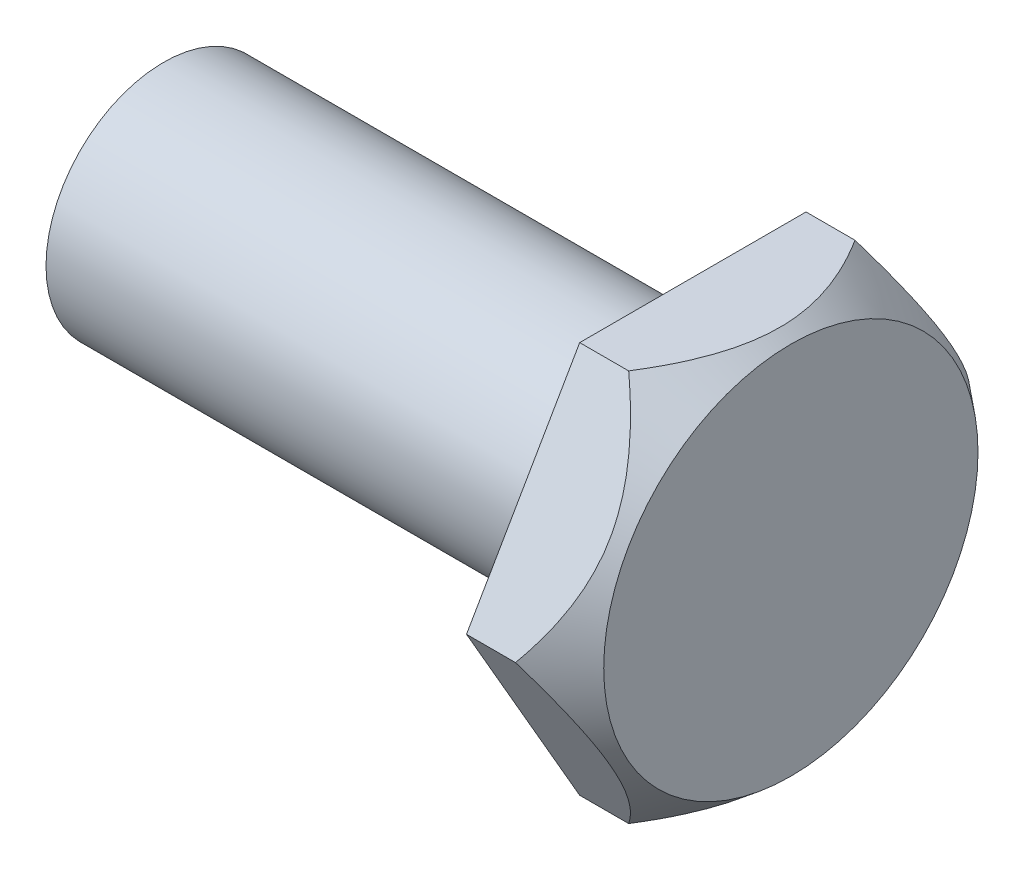
ISO-10303-21;
HEADER;
FILE_DESCRIPTION(('STEP AP214'),'2;1');
FILE_NAME('part.step','',(''),(''),'','','');
FILE_SCHEMA(('AUTOMOTIVE_DESIGN { 1 0 10303 214 1 1 1 1 }'));
ENDSEC;
DATA;
#1=APPLICATION_CONTEXT('core data for automotive mechanical design processes');
#2=APPLICATION_PROTOCOL_DEFINITION('international standard','automotive_design',2000,#1);
#3=PRODUCT_CONTEXT('',#1,'mechanical');
#4=PRODUCT('Part','Part','',(#3));
#5=PRODUCT_RELATED_PRODUCT_CATEGORY('part','',(#4));
#6=PRODUCT_DEFINITION_FORMATION('','',#4);
#7=PRODUCT_DEFINITION_CONTEXT('part definition',#1,'design');
#8=PRODUCT_DEFINITION('design','',#6,#7);
#9=PRODUCT_DEFINITION_SHAPE('','',#8);
#10=(LENGTH_UNIT() NAMED_UNIT(*) SI_UNIT(.MILLI.,.METRE.));
#11=(NAMED_UNIT(*) PLANE_ANGLE_UNIT() SI_UNIT($,.RADIAN.));
#12=(NAMED_UNIT(*) SI_UNIT($,.STERADIAN.) SOLID_ANGLE_UNIT());
#13=UNCERTAINTY_MEASURE_WITH_UNIT(LENGTH_MEASURE(1.E-05),#10,'distance_accuracy_value','');
#14=(GEOMETRIC_REPRESENTATION_CONTEXT(3) GLOBAL_UNCERTAINTY_ASSIGNED_CONTEXT((#13)) GLOBAL_UNIT_ASSIGNED_CONTEXT((#10,
#11,#12)) REPRESENTATION_CONTEXT('',''));
#15=CARTESIAN_POINT('',(0.,0.,0.));
#16=DIRECTION('',(0.,0.,1.));
#17=DIRECTION('',(1.,0.,0.));
#18=AXIS2_PLACEMENT_3D('',#15,#16,#17);
#19=CARTESIAN_POINT('',(5.,-9.99999999999994,-5.77350269189638));
#20=DIRECTION('',(0.,0.499999999999995,0.866025403784442));
#21=DIRECTION('',(0.,-0.866025403784442,0.499999999999995));
#22=AXIS2_PLACEMENT_3D('',#19,#20,#21);
#23=PLANE('',#22);
#24=CARTESIAN_POINT('',(2.49985566026766,-10.0001999999999,-5.77338722184254));
#25=CARTESIAN_POINT('',(2.60208467518783,-9.85852686353924,-5.85518224531506));
#26=CARTESIAN_POINT('',(2.70200639497535,-9.71558292882775,-5.93771096449977));
#27=CARTESIAN_POINT('',(2.89651431417004,-9.4269143562069,-6.104373842609));
#28=CARTESIAN_POINT('',(2.99109805277837,-9.28118847658979,-6.18850871843383));
#29=CARTESIAN_POINT('',(3.17470392595501,-8.98589768304951,-6.35899493757353));
#30=CARTESIAN_POINT('',(3.26368628893194,-8.83631408022678,-6.44535707092958));
#31=CARTESIAN_POINT('',(3.43446296157987,-8.53414647021996,-6.6198136219074));
#32=CARTESIAN_POINT('',(3.51625815008562,-8.38156283267477,-6.70790782611805));
#33=CARTESIAN_POINT('',(3.75045112758238,-7.91690475517259,-6.97617829224507));
#34=CARTESIAN_POINT('',(3.89039553403278,-7.59990272498793,-7.15919949970583));
#35=CARTESIAN_POINT('',(4.06799913309065,-7.1160294270294,-7.43856387853586));
#36=CARTESIAN_POINT('',(4.12177377354539,-6.95352485751446,-7.53238593548985));
#37=CARTESIAN_POINT('',(4.21746692388596,-6.62593053507777,-7.72152260573366));
#38=CARTESIAN_POINT('',(4.25938815721112,-6.46084138520395,-7.8168368708536));
#39=CARTESIAN_POINT('',(4.33871032958248,-6.08911976471419,-8.03145044850696));
#40=CARTESIAN_POINT('',(4.37267748881161,-5.88192616358385,-8.15107372989393));
#41=CARTESIAN_POINT('',(4.41927948249989,-5.46569987173225,-8.39138209153825));
#42=CARTESIAN_POINT('',(4.43191113799902,-5.25666691161239,-8.51206732733295));
#43=CARTESIAN_POINT('',(4.43521434084648,-4.83984013132415,-8.75272238113781));
#44=CARTESIAN_POINT('',(4.42602965332971,-4.63204719513949,-8.87269168877972));
#45=CARTESIAN_POINT('',(4.38644510874876,-4.21800376920535,-9.11173977219899));
#46=CARTESIAN_POINT('',(4.35604439850546,-4.0117533418233,-9.23081851196849));
#47=CARTESIAN_POINT('',(4.26630141702067,-3.55618197525321,-9.49384276309281));
#48=CARTESIAN_POINT('',(4.20199147726657,-3.30759485824364,-9.63736460201536));
#49=CARTESIAN_POINT('',(4.04725502781986,-2.8165969751545,-9.92084236198841));
#50=CARTESIAN_POINT('',(3.95681699311202,-2.57418898612793,-10.0607966797066));
#51=CARTESIAN_POINT('',(3.75343720990721,-2.09504523404485,-10.3374304539523));
#52=CARTESIAN_POINT('',(3.64036752653577,-1.85835070482231,-10.4740861041146));
#53=CARTESIAN_POINT('',(3.39608726520655,-1.39222410263783,-10.7432044233623));
#54=CARTESIAN_POINT('',(3.26488079551853,-1.1627903994069,-10.8756680336838));
#55=CARTESIAN_POINT('',(3.02822583050869,-0.776777620154309,-11.098532615696));
#56=CARTESIAN_POINT('',(2.92644536946085,-0.618490041669188,-11.1899199917437));
#57=CARTESIAN_POINT('',(2.71725475169805,-0.306260702457589,-11.3701856847864));
#58=CARTESIAN_POINT('',(2.60989089909902,-0.152295714503421,-11.4590774120275));
#59=CARTESIAN_POINT('',(2.49985566026766,0.00019999999999962,-11.5471208538464));
#60=B_SPLINE_CURVE_WITH_KNOTS('',3,(#24,#25,#26,#27,#28,#29,#30,#31,#32,#33,#34,#35,#36,#37,#38,
#39,#40,#41,#42,#43,#44,#45,#46,#47,#48,#49,#50,#51,#52,#53,#54,#55,#56,#57,#58,#59),
.UNSPECIFIED.,.F.,.F.,(4,2,2,2,2,2,2,2,2,2,2,2,2,2,2,2,2,4),(0.,0.578726598225102,
1.15771784486318,1.74044053909011,2.32309187958723,3.49620252422061,4.08148401745194,
4.66663092690834,5.39064458743798,6.11476611547105,6.83412908628144,7.55352098715262,
8.43453361817369,9.31593545579789,10.2024681456462,11.0888003498481,11.7162856672066,
12.3392094455715),.UNSPECIFIED.);
#61=CARTESIAN_POINT('',(2.5,-9.99999999999994,-5.77350269189637));
#62=VERTEX_POINT('',#61);
#63=CARTESIAN_POINT('',(2.5,0.,-11.5470053837925));
#64=VERTEX_POINT('',#63);
#65=EDGE_CURVE('E145',#62,#64,#60,.T.);
#66=ORIENTED_EDGE('',*,*,#65,.F.);
#67=DIRECTION('',(-1.,0.,0.));
#68=VECTOR('',#67,1.);
#69=CARTESIAN_POINT('',(5.,-9.99999999999994,-5.77350269189638));
#70=LINE('',#69,#68);
#71=CARTESIAN_POINT('',(0.,-9.99999999999994,-5.77350269189638));
#72=VERTEX_POINT('',#71);
#73=EDGE_CURVE('E64',#62,#72,#70,.T.);
#74=ORIENTED_EDGE('',*,*,#73,.T.);
#75=DIRECTION('',(0.,0.866025403784442,-0.499999999999995));
#76=VECTOR('',#75,1.);
#77=CARTESIAN_POINT('',(0.,-9.99999999999994,-5.77350269189638));
#78=LINE('',#77,#76);
#79=CARTESIAN_POINT('',(0.,0.,-11.5470053837925));
#80=VERTEX_POINT('',#79);
#81=EDGE_CURVE('E137',#72,#80,#78,.T.);
#82=ORIENTED_EDGE('',*,*,#81,.T.);
#83=DIRECTION('',(-1.,0.,0.));
#84=VECTOR('',#83,1.);
#85=CARTESIAN_POINT('',(5.,0.,-11.5470053837925));
#86=LINE('',#85,#84);
#87=EDGE_CURVE('E43',#64,#80,#86,.T.);
#88=ORIENTED_EDGE('',*,*,#87,.F.);
#89=EDGE_LOOP('',(#66,#74,#82,#88));
#90=FACE_BOUND('',#89,.T.);
#91=ADVANCED_FACE('F39',(#90),#23,.F.);
#92=CARTESIAN_POINT('',(5.,0.,-11.5470053837925));
#93=DIRECTION('',(0.,-0.500000000000001,0.866025403784438));
#94=DIRECTION('',(0.,-0.866025403784438,-0.500000000000001));
#95=AXIS2_PLACEMENT_3D('',#92,#93,#94);
#96=PLANE('',#95);
#97=CARTESIAN_POINT('',(2.49985566026766,-0.000200000000000101,-11.5471208538464));
#98=CARTESIAN_POINT('',(2.60208467518784,0.141473136460705,-11.4653258303738));
#99=CARTESIAN_POINT('',(2.70200639497536,0.284417071172192,-11.3827971111891));
#100=CARTESIAN_POINT('',(2.89651431417006,0.57308564379305,-11.2161342330799));
#101=CARTESIAN_POINT('',(2.99109805277838,0.718811523410157,-11.1319993572551));
#102=CARTESIAN_POINT('',(3.17470392595503,1.01410231695044,-10.9615131381154));
#103=CARTESIAN_POINT('',(3.26368628893196,1.16368591977317,-10.8751510047593));
#104=CARTESIAN_POINT('',(3.43446296157989,1.46585352977999,-10.7006944537815));
#105=CARTESIAN_POINT('',(3.51625815008564,1.61843716732518,-10.6126002495708));
#106=CARTESIAN_POINT('',(3.75045112758241,2.08309524482737,-10.3443297834438));
#107=CARTESIAN_POINT('',(3.89039553403281,2.40009727501203,-10.161308575983));
#108=CARTESIAN_POINT('',(4.06799913309069,2.88397057297057,-9.881944197153));
#109=CARTESIAN_POINT('',(4.12177377354543,3.04647514248551,-9.78812214019901));
#110=CARTESIAN_POINT('',(4.217466923886,3.37406946492221,-9.59898546995518));
#111=CARTESIAN_POINT('',(4.25938815721117,3.53915861479603,-9.50367120483525));
#112=CARTESIAN_POINT('',(4.33871032958253,3.91088023528579,-9.28905762718188));
#113=CARTESIAN_POINT('',(4.37267748881166,4.11807383641612,-9.16943434579491));
#114=CARTESIAN_POINT('',(4.41927948249994,4.53430012826773,-8.92912598415059));
#115=CARTESIAN_POINT('',(4.43191113799907,4.74333308838758,-8.80844074835589));
#116=CARTESIAN_POINT('',(4.43521434084653,5.16015986867583,-8.56778569455102));
#117=CARTESIAN_POINT('',(4.42602965332976,5.36795280486048,-8.44781638690911));
#118=CARTESIAN_POINT('',(4.38644510874881,5.78199623079462,-8.20876830348984));
#119=CARTESIAN_POINT('',(4.35604439850552,5.98824665817666,-8.08968956372034));
#120=CARTESIAN_POINT('',(4.26630141702072,6.44381802474675,-7.82666531259602));
#121=CARTESIAN_POINT('',(4.20199147726662,6.69240514175632,-7.68314347367347));
#122=CARTESIAN_POINT('',(4.04725502781991,7.18340302484546,-7.39966571370041));
#123=CARTESIAN_POINT('',(3.95681699311207,7.42581101387203,-7.25971139598221));
#124=CARTESIAN_POINT('',(3.75343720990726,7.9049547659551,-6.98307762173652));
#125=CARTESIAN_POINT('',(3.64036752653582,8.14164929517764,-6.84642197157417));
#126=CARTESIAN_POINT('',(3.3960872652066,8.60777589736212,-6.57730365232652));
#127=CARTESIAN_POINT('',(3.26488079551859,8.83720960059305,-6.44484004200497));
#128=CARTESIAN_POINT('',(3.02822583050874,9.22322237984565,-6.22197545999284));
#129=CARTESIAN_POINT('',(2.92644536946089,9.38150995833078,-6.13058808394508));
#130=CARTESIAN_POINT('',(2.71725475169808,9.69373929754241,-5.95032239090235));
#131=CARTESIAN_POINT('',(2.60989089909903,9.84770428549659,-5.86143066366122));
#132=CARTESIAN_POINT('',(2.49985566026766,10.0002,-5.7733872218424));
#133=B_SPLINE_CURVE_WITH_KNOTS('',3,(#97,#98,#99,#100,#101,#102,#103,#104,#105,#106,#107,#108,
#109,#110,#111,#112,#113,#114,#115,#116,#117,#118,#119,#120,#121,#122,#123,#124,#125,#126,#127,
#128,#129,#130,#131,#132),.UNSPECIFIED.,.F.,.F.,(4,2,2,2,2,2,2,2,2,2,2,2,2,2,2,2,2,4),(0.,
0.578726598225111,1.1577178448632,1.74044053909014,2.32309187958726,3.49620252422066,
4.081484017452,4.66663092690841,5.39064458743805,6.11476611547112,6.83412908628151,
7.55352098715269,8.43453361817375,9.31593545579795,10.2024681456462,11.0888003498482,
11.7162856672067,12.3392094455717),.UNSPECIFIED.);
#134=CARTESIAN_POINT('',(2.5,10.,-5.77350269189624));
#135=VERTEX_POINT('',#134);
#136=EDGE_CURVE('E131',#64,#135,#133,.T.);
#137=ORIENTED_EDGE('',*,*,#136,.F.);
#138=ORIENTED_EDGE('',*,*,#87,.T.);
#139=DIRECTION('',(0.,0.866025403784438,0.500000000000001));
#140=VECTOR('',#139,1.);
#141=CARTESIAN_POINT('',(0.,0.,-11.5470053837925));
#142=LINE('',#141,#140);
#143=CARTESIAN_POINT('',(0.,10.,-5.77350269189624));
#144=VERTEX_POINT('',#143);
#145=EDGE_CURVE('E126',#80,#144,#142,.T.);
#146=ORIENTED_EDGE('',*,*,#145,.T.);
#147=DIRECTION('',(-1.,0.,0.));
#148=VECTOR('',#147,1.);
#149=CARTESIAN_POINT('',(5.,10.,-5.77350269189624));
#150=LINE('',#149,#148);
#151=EDGE_CURVE('E116',#135,#144,#150,.T.);
#152=ORIENTED_EDGE('',*,*,#151,.F.);
#153=EDGE_LOOP('',(#137,#138,#146,#152));
#154=FACE_BOUND('',#153,.T.);
#155=ADVANCED_FACE('F129',(#154),#96,.F.);
#156=CARTESIAN_POINT('',(5.,10.,-5.77350269189624));
#157=DIRECTION('',(0.,-1.,0.));
#158=DIRECTION('',(0.,0.,-1.));
#159=AXIS2_PLACEMENT_3D('',#156,#157,#158);
#160=PLANE('',#159);
#161=CARTESIAN_POINT('',(-8.35662706903642,10.0000000000001,-17.5882417575278));
#162=CARTESIAN_POINT('',(-7.97728774264987,10.0000000000001,-17.2391089345561));
#163=CARTESIAN_POINT('',(-7.59917023824418,10.0000000000001,-16.888638172075));
#164=CARTESIAN_POINT('',(-6.84592339805097,10.0000000000001,-16.1844494205654));
#165=CARTESIAN_POINT('',(-6.4707942720274,10.0000000000001,-15.8307312072743));
#166=CARTESIAN_POINT('',(-5.72329920958807,10.,-15.1187412536086));
#167=CARTESIAN_POINT('',(-5.3509411810078,10.,-14.7604611985171));
#168=CARTESIAN_POINT('',(-4.61061924843071,10.,-14.0394023341909));
#169=CARTESIAN_POINT('',(-4.24265522995826,10.,-13.6766236426619));
#170=CARTESIAN_POINT('',(-3.50698481181781,10.,-12.9405134735512));
#171=CARTESIAN_POINT('',(-3.1393549670149,10.,-12.5671053329458));
#172=CARTESIAN_POINT('',(-2.41108252260193,10.,-11.8135408542725));
#173=CARTESIAN_POINT('',(-2.05043969112774,10.,-11.4333847409411));
#174=CARTESIAN_POINT('',(-1.33839051853618,10.,-10.6650878734714));
#175=CARTESIAN_POINT('',(-0.986976669328572,10.,-10.2769540985743));
#176=CARTESIAN_POINT('',(-0.295851771817263,10.,-9.49043781030286));
#177=CARTESIAN_POINT('',(0.0438610505675598,10.,-9.09205686672108));
#178=CARTESIAN_POINT('',(0.607339330625165,10.,-8.40467587052712));
#179=CARTESIAN_POINT('',(0.835132848513796,10.,-8.11898389461643));
#180=CARTESIAN_POINT('',(1.28117912364746,10.,-7.54016134039821));
#181=CARTESIAN_POINT('',(1.49943087980217,10.,-7.24702998665042));
#182=CARTESIAN_POINT('',(1.92390022086966,10.,-6.65199419820068));
#183=CARTESIAN_POINT('',(2.13011400830235,10.,-6.35008703960652));
#184=CARTESIAN_POINT('',(2.52701179015707,10.,-5.73618278704565));
#185=CARTESIAN_POINT('',(2.71769748897819,10.,-5.42418680571781));
#186=CARTESIAN_POINT('',(3.05280570259878,10.,-4.83469068446123));
#187=CARTESIAN_POINT('',(3.19992926298762,10.,-4.55873561198774));
#188=CARTESIAN_POINT('',(3.47579299967202,10.,-3.99765646875701));
#189=CARTESIAN_POINT('',(3.60453166636243,10.,-3.71253164741337));
#190=CARTESIAN_POINT('',(3.8387515987253,10.,-3.13389541890926));
#191=CARTESIAN_POINT('',(3.94430995674006,10.,-2.84041559417784));
#192=CARTESIAN_POINT('',(4.12772031764736,10.,-2.24490150142743));
#193=CARTESIAN_POINT('',(4.20558602056865,10.,-1.94287154337203));
#194=CARTESIAN_POINT('',(4.31392399550829,10.,-1.40660042017346));
#195=CARTESIAN_POINT('',(4.35131898505701,10.,-1.17375444581952));
#196=CARTESIAN_POINT('',(4.40605033394989,10.,-0.705707397152917));
#197=CARTESIAN_POINT('',(4.42338948717618,10.,-0.47050665547711));
#198=CARTESIAN_POINT('',(4.43721854881449,10.,0.000395911575754617));
#199=CARTESIAN_POINT('',(4.43371867902631,10.,0.236097434604736));
#200=CARTESIAN_POINT('',(4.40605758957446,10.,0.706283855006258));
#201=CARTESIAN_POINT('',(4.38189519433181,10.,0.940768682392127));
#202=CARTESIAN_POINT('',(4.31417340982602,9.99999999999999,1.40551529862139));
#203=CARTESIAN_POINT('',(4.27072569970184,9.99999999999999,1.63579356640222));
#204=CARTESIAN_POINT('',(4.16615955139027,9.99999999999999,2.09231382275418));
#205=CARTESIAN_POINT('',(4.1050370725345,9.99999999999999,2.31855487579778));
#206=CARTESIAN_POINT('',(3.9670838088809,9.99999999999999,2.76646805689877));
#207=CARTESIAN_POINT('',(3.89023306874717,9.99999999999999,2.98813398298915));
#208=CARTESIAN_POINT('',(3.72298819408545,9.99999999999999,3.42624280728566));
#209=CARTESIAN_POINT('',(3.63259437104085,9.99999999999999,3.64268582548288));
#210=CARTESIAN_POINT('',(3.40888186338885,9.99999999999999,4.14008164597385));
#211=CARTESIAN_POINT('',(3.27117741048021,9.99999999999998,4.41905695199646));
#212=CARTESIAN_POINT('',(2.97942567580929,9.99999999999998,4.96838107495215));
#213=CARTESIAN_POINT('',(2.82537119433022,9.99999999999998,5.23872602278562));
#214=CARTESIAN_POINT('',(2.50391254127959,9.99999999999998,5.7719758553274));
#215=CARTESIAN_POINT('',(2.33648474477565,9.99999999999998,6.03486640976312));
#216=CARTESIAN_POINT('',(1.99111175713331,9.99999999999998,6.55355223906987));
#217=CARTESIAN_POINT('',(1.81316801950844,9.99999999999998,6.80934848736804));
#218=CARTESIAN_POINT('',(1.44673171699159,9.99999999999998,7.31752860399921));
#219=CARTESIAN_POINT('',(1.25814474063016,9.99999999999998,7.56984411339175));
#220=CARTESIAN_POINT('',(0.873829840215399,9.99999999999997,8.06896766590264));
#221=CARTESIAN_POINT('',(0.678101729330905,9.99999999999997,8.31577556465454));
#222=CARTESIAN_POINT('',(0.280957134366479,9.99999999999997,8.80434376141056));
#223=CARTESIAN_POINT('',(0.0795466103589055,9.99999999999997,9.04610891705088));
#224=CARTESIAN_POINT('',(-0.328183318593257,9.99999999999997,9.52546854557073));
#225=CARTESIAN_POINT('',(-0.534502903544672,9.99999999999997,9.76306286495601));
#226=CARTESIAN_POINT('',(-1.04494842355568,9.99999999999997,10.3406073190432));
#227=CARTESIAN_POINT('',(-1.35134375872624,9.99999999999997,10.6785507196934));
#228=CARTESIAN_POINT('',(-1.9709756821915,9.99999999999996,11.3481047128741));
#229=CARTESIAN_POINT('',(-2.28421252369331,9.99999999999996,11.6797150701615));
#230=CARTESIAN_POINT('',(-2.91635203293325,9.99999999999996,12.337808130985));
#231=CARTESIAN_POINT('',(-3.23525752273593,9.99999999999996,12.6642881188828));
#232=CARTESIAN_POINT('',(-3.87757020644268,9.99999999999996,13.3127893326489));
#233=CARTESIAN_POINT('',(-4.20097745572092,9.99999999999995,13.6348105035737));
#234=CARTESIAN_POINT('',(-4.83999412661594,9.99999999999995,14.2637274750938));
#235=CARTESIAN_POINT('',(-5.15547404837216,9.99999999999995,14.5707550365838));
#236=CARTESIAN_POINT('',(-5.78935532002772,9.99999999999995,15.1817824119234));
#237=CARTESIAN_POINT('',(-6.10775669613608,9.99999999999995,15.4857821985592));
#238=CARTESIAN_POINT('',(-6.74669312096204,9.99999999999995,16.0908355033313));
#239=CARTESIAN_POINT('',(-7.0672254987366,9.99999999999995,16.3918918449499));
#240=CARTESIAN_POINT('',(-7.71041486444918,9.99999999999994,16.9917064317293));
#241=CARTESIAN_POINT('',(-8.03307178396953,9.99999999999994,17.2904647502292));
#242=CARTESIAN_POINT('',(-8.35662706903642,9.99999999999994,17.5882417575279));
#243=B_SPLINE_CURVE_WITH_KNOTS('',3,(#161,#162,#163,#164,#165,#166,#167,#168,#169,#170,#171,
#172,#173,#174,#175,#176,#177,#178,#179,#180,#181,#182,#183,#184,#185,#186,#187,#188,#189,#190,
#191,#192,#193,#194,#195,#196,#197,#198,#199,#200,#201,#202,#203,#204,#205,#206,#207,#208,#209,
#210,#211,#212,#213,#214,#215,#216,#217,#218,#219,#220,#221,#222,#223,#224,#225,#226,#227,#228,
#229,#230,#231,#232,#233,#234,#235,#236,#237,#238,#239,#240,#241,#242),.UNSPECIFIED.,.F.,.F.,(4,
2,2,2,2,2,2,2,2,2,2,2,2,2,2,2,2,2,2,2,2,2,2,2,2,2,2,2,2,2,2,2,2,2,2,2,2,2,2,2,4),(0.,
1.54665805225938,3.09342372941361,4.64359691339925,6.19372962276105,7.7656852884161,
9.33758869903942,10.9081709990313,12.4785141134674,13.5745278278695,14.6706562578265,
15.7671286227889,16.8634804737197,17.8011113362478,18.7388191445309,19.6733594653186,
20.6074368078336,21.3141402405969,22.0207452140419,22.727003617527,23.4333022057311,
24.1355629998527,24.8379844664794,25.5413027222289,26.244604804531,27.1772291450048,
28.1102658830341,29.0449889881248,29.979583196587,30.9244446421433,31.8693308255509,
32.8132603206112,33.7572244814476,35.1255826710275,36.4939915902383,37.8631019732006,
39.2322292118992,40.552865604745,41.8735138569189,43.192738059353,44.5119199839387),.UNSPECIFIED.);
#244=CARTESIAN_POINT('',(2.5,9.99999999999998,5.77350269189631));
#245=VERTEX_POINT('',#244);
#246=EDGE_CURVE('E98',#135,#245,#243,.T.);
#247=ORIENTED_EDGE('',*,*,#246,.F.);
#248=ORIENTED_EDGE('',*,*,#151,.T.);
#249=DIRECTION('',(0.,0.,1.));
#250=VECTOR('',#249,1.);
#251=CARTESIAN_POINT('',(0.,10.,-5.77350269189624));
#252=LINE('',#251,#250);
#253=CARTESIAN_POINT('',(0.,9.99999999999998,5.77350269189631));
#254=VERTEX_POINT('',#253);
#255=EDGE_CURVE('E140',#144,#254,#252,.T.);
#256=ORIENTED_EDGE('',*,*,#255,.T.);
#257=DIRECTION('',(-1.,0.,0.));
#258=VECTOR('',#257,1.);
#259=CARTESIAN_POINT('',(5.,9.99999999999998,5.77350269189631));
#260=LINE('',#259,#258);
#261=EDGE_CURVE('E112',#245,#254,#260,.T.);
#262=ORIENTED_EDGE('',*,*,#261,.F.);
#263=EDGE_LOOP('',(#247,#248,#256,#262));
#264=FACE_BOUND('',#263,.T.);
#265=ADVANCED_FACE('F201',(#264),#160,.F.);
#266=CARTESIAN_POINT('',(5.,9.99999999999998,5.77350269189631));
#267=DIRECTION('',(0.,-0.499999999999995,-0.866025403784442));
#268=DIRECTION('',(0.,0.866025403784442,-0.499999999999995));
#269=AXIS2_PLACEMENT_3D('',#266,#267,#268);
#270=PLANE('',#269);
#271=CARTESIAN_POINT('',(2.49985566026766,10.0002,5.77338722184247));
#272=CARTESIAN_POINT('',(2.60208467518784,9.85852686353928,5.855182245315));
#273=CARTESIAN_POINT('',(2.70200639497535,9.71558292882779,5.9377109644997));
#274=CARTESIAN_POINT('',(2.89651431417006,9.42691435620693,6.10437384260893));
#275=CARTESIAN_POINT('',(2.99109805277838,9.28118847658982,6.18850871843376));
#276=CARTESIAN_POINT('',(3.17470392595502,8.98589768304953,6.35899493757346));
#277=CARTESIAN_POINT('',(3.26368628893196,8.83631408022681,6.44535707092952));
#278=CARTESIAN_POINT('',(3.43446296157989,8.53414647021998,6.61981362190734));
#279=CARTESIAN_POINT('',(3.51625815008564,8.3815628326748,6.70790782611799));
#280=CARTESIAN_POINT('',(3.75045112758241,7.9169047551726,6.97617829224501));
#281=CARTESIAN_POINT('',(3.89039553403281,7.59990272498794,7.15919949970578));
#282=CARTESIAN_POINT('',(4.06799913309069,7.11602942702941,7.43856387853581));
#283=CARTESIAN_POINT('',(4.12177377354543,6.95352485751446,7.5323859354898));
#284=CARTESIAN_POINT('',(4.217466923886,6.62593053507777,7.72152260573362));
#285=CARTESIAN_POINT('',(4.25938815721116,6.46084138520394,7.81683687085356));
#286=CARTESIAN_POINT('',(4.33871032958253,6.08911976471418,8.03145044850692));
#287=CARTESIAN_POINT('',(4.37267748881166,5.88192616358385,8.15107372989389));
#288=CARTESIAN_POINT('',(4.41927948249994,5.46569987173224,8.3913820915382));
#289=CARTESIAN_POINT('',(4.43191113799907,5.25666691161239,8.51206732733291));
#290=CARTESIAN_POINT('',(4.43521434084653,4.83984013132414,8.75272238113777));
#291=CARTESIAN_POINT('',(4.42602965332976,4.63204719513949,8.87269168877968));
#292=CARTESIAN_POINT('',(4.38644510874881,4.21800376920535,9.11173977219895));
#293=CARTESIAN_POINT('',(4.35604439850552,4.0117533418233,9.23081851196844));
#294=CARTESIAN_POINT('',(4.26630141702072,3.55618197525321,9.49384276309277));
#295=CARTESIAN_POINT('',(4.20199147726662,3.30759485824364,9.63736460201532));
#296=CARTESIAN_POINT('',(4.04725502781991,2.81659697515451,9.92084236198836));
#297=CARTESIAN_POINT('',(3.95681699311208,2.57418898612793,10.0607966797066));
#298=CARTESIAN_POINT('',(3.75343720990727,2.09504523404486,10.3374304539523));
#299=CARTESIAN_POINT('',(3.64036752653583,1.85835070482232,10.4740861041146));
#300=CARTESIAN_POINT('',(3.39608726520661,1.39222410263784,10.7432044233622));
#301=CARTESIAN_POINT('',(3.26488079551859,1.16279039940691,10.8756680336838));
#302=CARTESIAN_POINT('',(3.02822583050874,0.776777620154306,11.0985326156959));
#303=CARTESIAN_POINT('',(2.92644536946089,0.618490041669168,11.1899199917437));
#304=CARTESIAN_POINT('',(2.71725475169808,0.306260702457537,11.3701856847864));
#305=CARTESIAN_POINT('',(2.60989089909903,0.152295714503355,11.4590774120275));
#306=CARTESIAN_POINT('',(2.49985566026766,-0.000200000000078887,11.5471208538464));
#307=B_SPLINE_CURVE_WITH_KNOTS('',3,(#271,#272,#273,#274,#275,#276,#277,#278,#279,#280,#281,
#282,#283,#284,#285,#286,#287,#288,#289,#290,#291,#292,#293,#294,#295,#296,#297,#298,#299,#300,
#301,#302,#303,#304,#305,#306),.UNSPECIFIED.,.F.,.F.,(4,2,2,2,2,2,2,2,2,2,2,2,2,2,2,2,2,4),(0.,
0.578726598225112,1.1577178448632,1.74044053909014,2.32309187958726,3.49620252422066,
4.081484017452,4.66663092690841,5.39064458743804,6.11476611547111,6.83412908628151,
7.55352098715268,8.43453361817375,9.31593545579794,10.2024681456462,11.0888003498482,
11.7162856672067,12.3392094455717),.UNSPECIFIED.);
#308=CARTESIAN_POINT('',(2.5,0.,11.5470053837925));
#309=VERTEX_POINT('',#308);
#310=EDGE_CURVE('E94',#245,#309,#307,.T.);
#311=ORIENTED_EDGE('',*,*,#310,.F.);
#312=ORIENTED_EDGE('',*,*,#261,.T.);
#313=DIRECTION('',(0.,-0.866025403784442,0.499999999999995));
#314=VECTOR('',#313,1.);
#315=CARTESIAN_POINT('',(0.,9.99999999999998,5.77350269189631));
#316=LINE('',#315,#314);
#317=CARTESIAN_POINT('',(0.,0.,11.5470053837925));
#318=VERTEX_POINT('',#317);
#319=EDGE_CURVE('E115',#254,#318,#316,.T.);
#320=ORIENTED_EDGE('',*,*,#319,.T.);
#321=DIRECTION('',(-1.,0.,0.));
#322=VECTOR('',#321,1.);
#323=CARTESIAN_POINT('',(5.,0.,11.5470053837925));
#324=LINE('',#323,#322);
#325=EDGE_CURVE('E102',#309,#318,#324,.T.);
#326=ORIENTED_EDGE('',*,*,#325,.F.);
#327=EDGE_LOOP('',(#311,#312,#320,#326));
#328=FACE_BOUND('',#327,.T.);
#329=ADVANCED_FACE('F109',(#328),#270,.F.);
#330=CARTESIAN_POINT('',(5.,0.,11.5470053837925));
#331=DIRECTION('',(0.,0.500000000000007,-0.866025403784435));
#332=DIRECTION('',(0.,0.866025403784435,0.500000000000007));
#333=AXIS2_PLACEMENT_3D('',#330,#331,#332);
#334=PLANE('',#333);
#335=CARTESIAN_POINT('',(2.49985566026766,0.000199999999919467,11.5471208538464));
#336=CARTESIAN_POINT('',(2.60208467518784,-0.141473136460786,11.4653258303738));
#337=CARTESIAN_POINT('',(2.70200639497535,-0.284417071172273,11.3827971111891));
#338=CARTESIAN_POINT('',(2.89651431417006,-0.573085643793129,11.2161342330799));
#339=CARTESIAN_POINT('',(2.99109805277838,-0.718811523410235,11.1319993572551));
#340=CARTESIAN_POINT('',(3.17470392595503,-1.01410231695052,10.9615131381154));
#341=CARTESIAN_POINT('',(3.26368628893196,-1.16368591977324,10.8751510047593));
#342=CARTESIAN_POINT('',(3.43446296157989,-1.46585352978007,10.7006944537815));
#343=CARTESIAN_POINT('',(3.51625815008564,-1.61843716732525,10.6126002495708));
#344=CARTESIAN_POINT('',(3.75045112758241,-2.08309524482744,10.3443297834438));
#345=CARTESIAN_POINT('',(3.89039553403281,-2.4000972750121,10.161308575983));
#346=CARTESIAN_POINT('',(4.06799913309069,-2.88397057297063,9.88194419715298));
#347=CARTESIAN_POINT('',(4.12177377354543,-3.04647514248557,9.78812214019899));
#348=CARTESIAN_POINT('',(4.217466923886,-3.37406946492227,9.59898546995516));
#349=CARTESIAN_POINT('',(4.25938815721116,-3.53915861479609,9.50367120483522));
#350=CARTESIAN_POINT('',(4.33871032958253,-3.91088023528585,9.28905762718185));
#351=CARTESIAN_POINT('',(4.37267748881166,-4.11807383641618,9.16943434579489));
#352=CARTESIAN_POINT('',(4.41927948249994,-4.53430012826778,8.92912598415056));
#353=CARTESIAN_POINT('',(4.43191113799907,-4.74333308838764,8.80844074835586));
#354=CARTESIAN_POINT('',(4.43521434084653,-5.16015986867588,8.56778569455099));
#355=CARTESIAN_POINT('',(4.42602965332976,-5.36795280486053,8.44781638690907));
#356=CARTESIAN_POINT('',(4.38644510874881,-5.78199623079467,8.2087683034898));
#357=CARTESIAN_POINT('',(4.35604439850551,-5.98824665817671,8.0896895637203));
#358=CARTESIAN_POINT('',(4.26630141702072,-6.4438180247468,7.82666531259598));
#359=CARTESIAN_POINT('',(4.20199147726662,-6.69240514175636,7.68314347367343));
#360=CARTESIAN_POINT('',(4.04725502781991,-7.1834030248455,7.39966571370037));
#361=CARTESIAN_POINT('',(3.95681699311208,-7.42581101387207,7.25971139598216));
#362=CARTESIAN_POINT('',(3.75343720990727,-7.90495476595514,6.98307762173647));
#363=CARTESIAN_POINT('',(3.64036752653583,-8.14164929517768,6.84642197157412));
#364=CARTESIAN_POINT('',(3.39608726520661,-8.60777589736215,6.57730365232647));
#365=CARTESIAN_POINT('',(3.26488079551859,-8.83720960059308,6.44484004200492));
#366=CARTESIAN_POINT('',(3.02822583050875,-9.22322237984568,6.22197545999279));
#367=CARTESIAN_POINT('',(2.92644536946089,-9.38150995833082,6.13058808394502));
#368=CARTESIAN_POINT('',(2.71725475169808,-9.69373929754244,5.95032239090228));
#369=CARTESIAN_POINT('',(2.60989089909903,-9.84770428549663,5.86143066366115));
#370=CARTESIAN_POINT('',(2.49985566026766,-10.0002000000001,5.77338722184233));
#371=B_SPLINE_CURVE_WITH_KNOTS('',3,(#335,#336,#337,#338,#339,#340,#341,#342,#343,#344,#345,
#346,#347,#348,#349,#350,#351,#352,#353,#354,#355,#356,#357,#358,#359,#360,#361,#362,#363,#364,
#365,#366,#367,#368,#369,#370),.UNSPECIFIED.,.F.,.F.,(4,2,2,2,2,2,2,2,2,2,2,2,2,2,2,2,2,4),(0.,
0.578726598225111,1.1577178448632,1.74044053909014,2.32309187958726,3.49620252422066,
4.081484017452,4.66663092690841,5.39064458743804,6.11476611547111,6.8341290862815,
7.55352098715268,8.43453361817375,9.31593545579793,10.2024681456462,11.0888003498482,
11.7162856672067,12.3392094455717),.UNSPECIFIED.);
#372=CARTESIAN_POINT('',(2.5,-10.0000000000001,5.77350269189617));
#373=VERTEX_POINT('',#372);
#374=EDGE_CURVE('E54',#309,#373,#371,.T.);
#375=ORIENTED_EDGE('',*,*,#374,.F.);
#376=ORIENTED_EDGE('',*,*,#325,.T.);
#377=DIRECTION('',(0.,-0.866025403784435,-0.500000000000007));
#378=VECTOR('',#377,1.);
#379=CARTESIAN_POINT('',(0.,0.,11.5470053837925));
#380=LINE('',#379,#378);
#381=CARTESIAN_POINT('',(0.,-10.0000000000001,5.77350269189617));
#382=VERTEX_POINT('',#381);
#383=EDGE_CURVE('E150',#318,#382,#380,.T.);
#384=ORIENTED_EDGE('',*,*,#383,.T.);
#385=DIRECTION('',(-1.,0.,0.));
#386=VECTOR('',#385,1.);
#387=CARTESIAN_POINT('',(5.,-10.0000000000001,5.77350269189617));
#388=LINE('',#387,#386);
#389=EDGE_CURVE('E110',#373,#382,#388,.T.);
#390=ORIENTED_EDGE('',*,*,#389,.F.);
#391=EDGE_LOOP('',(#375,#376,#384,#390));
#392=FACE_BOUND('',#391,.T.);
#393=ADVANCED_FACE('F101',(#392),#334,.F.);
#394=CARTESIAN_POINT('',(5.,-10.0000000000001,5.77350269189617));
#395=DIRECTION('',(0.,1.,0.));
#396=DIRECTION('',(0.,0.,1.));
#397=AXIS2_PLACEMENT_3D('',#394,#395,#396);
#398=PLANE('',#397);
#399=CARTESIAN_POINT('',(-8.35662706903642,-10.0000000000002,17.5882417575277));
#400=CARTESIAN_POINT('',(-7.97728774264988,-10.0000000000002,17.239108934556));
#401=CARTESIAN_POINT('',(-7.59917023824419,-10.0000000000002,16.8886381720749));
#402=CARTESIAN_POINT('',(-6.84592339805097,-10.0000000000002,16.1844494205654));
#403=CARTESIAN_POINT('',(-6.4707942720274,-10.0000000000002,15.8307312072742));
#404=CARTESIAN_POINT('',(-5.72329920958807,-10.0000000000002,15.1187412536086));
#405=CARTESIAN_POINT('',(-5.3509411810078,-10.0000000000002,14.760461198517));
#406=CARTESIAN_POINT('',(-4.61061924843071,-10.0000000000001,14.0394023341909));
#407=CARTESIAN_POINT('',(-4.24265522995826,-10.0000000000001,13.6766236426618));
#408=CARTESIAN_POINT('',(-3.50698481181781,-10.0000000000001,12.9405134735512));
#409=CARTESIAN_POINT('',(-3.1393549670149,-10.0000000000001,12.5671053329457));
#410=CARTESIAN_POINT('',(-2.41108252260193,-10.0000000000001,11.8135408542724));
#411=CARTESIAN_POINT('',(-2.05043969112774,-10.0000000000001,11.433384740941));
#412=CARTESIAN_POINT('',(-1.33839051853618,-10.0000000000001,10.6650878734713));
#413=CARTESIAN_POINT('',(-0.986976669328575,-10.0000000000001,10.2769540985742));
#414=CARTESIAN_POINT('',(-0.295851771817264,-10.0000000000001,9.49043781030279));
#415=CARTESIAN_POINT('',(0.0438610505675585,-10.0000000000001,9.09205686672101));
#416=CARTESIAN_POINT('',(0.607339330625163,-10.0000000000001,8.40467587052705));
#417=CARTESIAN_POINT('',(0.835132848513793,-10.0000000000001,8.11898389461636));
#418=CARTESIAN_POINT('',(1.28117912364746,-10.0000000000001,7.54016134039814));
#419=CARTESIAN_POINT('',(1.49943087980217,-10.0000000000001,7.24702998665035));
#420=CARTESIAN_POINT('',(1.92390022086966,-10.0000000000001,6.65199419820061));
#421=CARTESIAN_POINT('',(2.13011400830235,-10.0000000000001,6.35008703960645));
#422=CARTESIAN_POINT('',(2.52701179015707,-10.0000000000001,5.73618278704558));
#423=CARTESIAN_POINT('',(2.71769748897819,-10.0000000000001,5.42418680571774));
#424=CARTESIAN_POINT('',(3.05280570259878,-10.,4.83469068446116));
#425=CARTESIAN_POINT('',(3.19992926298762,-10.,4.55873561198767));
#426=CARTESIAN_POINT('',(3.47579299967202,-10.,3.99765646875694));
#427=CARTESIAN_POINT('',(3.60453166636243,-10.,3.7125316474133));
#428=CARTESIAN_POINT('',(3.8387515987253,-10.,3.13389541890919));
#429=CARTESIAN_POINT('',(3.94430995674006,-10.,2.84041559417777));
#430=CARTESIAN_POINT('',(4.12772031764736,-10.,2.24490150142736));
#431=CARTESIAN_POINT('',(4.20558602056865,-10.,1.94287154337196));
#432=CARTESIAN_POINT('',(4.31392399550829,-10.,1.40660042017339));
#433=CARTESIAN_POINT('',(4.351318985057,-10.,1.17375444581945));
#434=CARTESIAN_POINT('',(4.40605033394989,-10.,0.705707397152846));
#435=CARTESIAN_POINT('',(4.42338948717618,-10.,0.470506655477039));
#436=CARTESIAN_POINT('',(4.43721854881448,-10.,-0.000395911575825579));
#437=CARTESIAN_POINT('',(4.4337186790263,-10.,-0.236097434604808));
#438=CARTESIAN_POINT('',(4.40605758957446,-9.99999999999999,-0.706283855006331));
#439=CARTESIAN_POINT('',(4.38189519433181,-9.99999999999999,-0.940768682392199));
#440=CARTESIAN_POINT('',(4.31417340982601,-9.99999999999998,-1.40551529862147));
#441=CARTESIAN_POINT('',(4.27072569970184,-9.99999999999998,-1.6357935664023));
#442=CARTESIAN_POINT('',(4.16615955139027,-9.99999999999998,-2.09231382275425));
#443=CARTESIAN_POINT('',(4.1050370725345,-9.99999999999998,-2.31855487579785));
#444=CARTESIAN_POINT('',(3.9670838088809,-9.99999999999997,-2.76646805689884));
#445=CARTESIAN_POINT('',(3.89023306874716,-9.99999999999997,-2.98813398298922));
#446=CARTESIAN_POINT('',(3.72298819408544,-9.99999999999997,-3.42624280728573));
#447=CARTESIAN_POINT('',(3.63259437104085,-9.99999999999996,-3.64268582548295));
#448=CARTESIAN_POINT('',(3.40888186338885,-9.99999999999996,-4.14008164597392));
#449=CARTESIAN_POINT('',(3.2711774104802,-9.99999999999995,-4.41905695199654));
#450=CARTESIAN_POINT('',(2.97942567580928,-9.99999999999995,-4.96838107495222));
#451=CARTESIAN_POINT('',(2.82537119433022,-9.99999999999995,-5.23872602278569));
#452=CARTESIAN_POINT('',(2.50391254127959,-9.99999999999994,-5.77197585532747));
#453=CARTESIAN_POINT('',(2.33648474477565,-9.99999999999994,-6.03486640976319));
#454=CARTESIAN_POINT('',(1.99111175713331,-9.99999999999993,-6.55355223906995));
#455=CARTESIAN_POINT('',(1.81316801950844,-9.99999999999993,-6.80934848736812));
#456=CARTESIAN_POINT('',(1.44673171699159,-9.99999999999993,-7.31752860399928));
#457=CARTESIAN_POINT('',(1.25814474063016,-9.99999999999992,-7.56984411339182));
#458=CARTESIAN_POINT('',(0.873829840215395,-9.99999999999992,-8.06896766590272));
#459=CARTESIAN_POINT('',(0.678101729330902,-9.99999999999991,-8.31577556465462));
#460=CARTESIAN_POINT('',(0.280957134366474,-9.99999999999991,-8.80434376141064));
#461=CARTESIAN_POINT('',(0.0795466103588979,-9.99999999999991,-9.04610891705096));
#462=CARTESIAN_POINT('',(-0.328183318593265,-9.9999999999999,-9.52546854557081));
#463=CARTESIAN_POINT('',(-0.534502903544678,-9.9999999999999,-9.76306286495609));
#464=CARTESIAN_POINT('',(-1.04494842355569,-9.9999999999999,-10.3406073190433));
#465=CARTESIAN_POINT('',(-1.35134375872625,-9.99999999999989,-10.6785507196935));
#466=CARTESIAN_POINT('',(-1.97097568219151,-9.99999999999988,-11.3481047128741));
#467=CARTESIAN_POINT('',(-2.28421252369331,-9.99999999999988,-11.6797150701616));
#468=CARTESIAN_POINT('',(-2.91635203293326,-9.99999999999987,-12.337808130985));
#469=CARTESIAN_POINT('',(-3.23525752273593,-9.99999999999987,-12.6642881188829));
#470=CARTESIAN_POINT('',(-3.87757020644268,-9.99999999999986,-13.3127893326489));
#471=CARTESIAN_POINT('',(-4.20097745572092,-9.99999999999986,-13.6348105035738));
#472=CARTESIAN_POINT('',(-4.83999412661594,-9.99999999999985,-14.2637274750939));
#473=CARTESIAN_POINT('',(-5.15547404837215,-9.99999999999985,-14.5707550365838));
#474=CARTESIAN_POINT('',(-5.78935532002772,-9.99999999999984,-15.1817824119235));
#475=CARTESIAN_POINT('',(-6.10775669613608,-9.99999999999984,-15.4857821985593));
#476=CARTESIAN_POINT('',(-6.74669312096204,-9.99999999999983,-16.0908355033314));
#477=CARTESIAN_POINT('',(-7.06722549873661,-9.99999999999983,-16.39189184495));
#478=CARTESIAN_POINT('',(-7.71041486444919,-9.99999999999982,-16.9917064317294));
#479=CARTESIAN_POINT('',(-8.03307178396954,-9.99999999999982,-17.2904647502293));
#480=CARTESIAN_POINT('',(-8.35662706903642,-9.99999999999982,-17.5882417575279));
#481=B_SPLINE_CURVE_WITH_KNOTS('',3,(#399,#400,#401,#402,#403,#404,#405,#406,#407,#408,#409,
#410,#411,#412,#413,#414,#415,#416,#417,#418,#419,#420,#421,#422,#423,#424,#425,#426,#427,#428,
#429,#430,#431,#432,#433,#434,#435,#436,#437,#438,#439,#440,#441,#442,#443,#444,#445,#446,#447,
#448,#449,#450,#451,#452,#453,#454,#455,#456,#457,#458,#459,#460,#461,#462,#463,#464,#465,#466,
#467,#468,#469,#470,#471,#472,#473,#474,#475,#476,#477,#478,#479,#480),.UNSPECIFIED.,.F.,.F.,(4,
2,2,2,2,2,2,2,2,2,2,2,2,2,2,2,2,2,2,2,2,2,2,2,2,2,2,2,2,2,2,2,2,2,2,2,2,2,2,2,4),(0.,
1.54665805225937,3.09342372941361,4.64359691339924,6.19372962276105,7.7656852884161,
9.33758869903941,10.9081709990313,12.4785141134674,13.5745278278695,14.6706562578265,
15.7671286227889,16.8634804737197,17.8011113362478,18.7388191445309,19.6733594653186,
20.6074368078336,21.3141402405969,22.0207452140419,22.727003617527,23.4333022057311,
24.1355629998527,24.8379844664794,25.5413027222289,26.244604804531,27.1772291450048,
28.1102658830341,29.0449889881248,29.979583196587,30.9244446421434,31.869330825551,
32.8132603206112,33.7572244814476,35.1255826710275,36.4939915902383,37.8631019732006,
39.2322292118992,40.552865604745,41.8735138569189,43.192738059353,44.5119199839387),.UNSPECIFIED.);
#482=EDGE_CURVE('E108',#373,#62,#481,.T.);
#483=ORIENTED_EDGE('',*,*,#482,.F.);
#484=ORIENTED_EDGE('',*,*,#389,.T.);
#485=DIRECTION('',(0.,0.,-1.));
#486=VECTOR('',#485,1.);
#487=CARTESIAN_POINT('',(0.,-10.0000000000001,5.77350269189617));
#488=LINE('',#487,#486);
#489=EDGE_CURVE('E146',#382,#72,#488,.T.);
#490=ORIENTED_EDGE('',*,*,#489,.T.);
#491=ORIENTED_EDGE('',*,*,#73,.F.);
#492=EDGE_LOOP('',(#483,#484,#490,#491));
#493=FACE_BOUND('',#492,.T.);
#494=ADVANCED_FACE('F151',(#493),#398,.F.);
#495=CARTESIAN_POINT('',(0.,0.,0.));
#496=DIRECTION('',(1.,0.,0.));
#497=DIRECTION('',(0.,0.,-1.));
#498=AXIS2_PLACEMENT_3D('',#495,#496,#497);
#499=PLANE('',#498);
#500=CARTESIAN_POINT('',(0.,0.,0.));
#501=DIRECTION('',(-1.,0.,0.));
#502=DIRECTION('',(0.,0.,1.));
#503=AXIS2_PLACEMENT_3D('',#500,#501,#502);
#504=CIRCLE('',#503,6.);
#505=CARTESIAN_POINT('',(0.,0.,6.));
#506=VERTEX_POINT('',#505);
#507=EDGE_CURVE('E11',#506,#506,#504,.T.);
#508=ORIENTED_EDGE('',*,*,#507,.F.);
#509=EDGE_LOOP('',(#508));
#510=FACE_BOUND('',#509,.T.);
#511=ORIENTED_EDGE('',*,*,#81,.F.);
#512=ORIENTED_EDGE('',*,*,#489,.F.);
#513=ORIENTED_EDGE('',*,*,#383,.F.);
#514=ORIENTED_EDGE('',*,*,#319,.F.);
#515=ORIENTED_EDGE('',*,*,#255,.F.);
#516=ORIENTED_EDGE('',*,*,#145,.F.);
#517=EDGE_LOOP('',(#511,#512,#513,#514,#515,#516));
#518=FACE_BOUND('',#517,.T.);
#519=ADVANCED_FACE('F133',(#510,#518),#499,.F.);
#520=CARTESIAN_POINT('',(-27.,0.,0.));
#521=DIRECTION('',(1.,0.,0.));
#522=DIRECTION('',(0.,0.,-1.));
#523=AXIS2_PLACEMENT_3D('',#520,#521,#522);
#524=CYLINDRICAL_SURFACE('',#523,6.);
#525=CARTESIAN_POINT('',(-27.,0.,0.));
#526=DIRECTION('',(-1.,0.,0.));
#527=DIRECTION('',(0.,0.,1.));
#528=AXIS2_PLACEMENT_3D('',#525,#526,#527);
#529=CIRCLE('',#528,6.);
#530=CARTESIAN_POINT('',(-27.,0.,6.));
#531=VERTEX_POINT('',#530);
#532=EDGE_CURVE('E136',#531,#531,#529,.T.);
#533=ORIENTED_EDGE('',*,*,#532,.F.);
#534=EDGE_LOOP('',(#533));
#535=FACE_BOUND('',#534,.T.);
#536=ORIENTED_EDGE('',*,*,#507,.T.);
#537=EDGE_LOOP('',(#536));
#538=FACE_BOUND('',#537,.T.);
#539=ADVANCED_FACE('F258',(#535,#538),#524,.T.);
#540=CARTESIAN_POINT('',(-27.,0.,0.));
#541=DIRECTION('',(-1.,0.,0.));
#542=DIRECTION('',(0.,0.,1.));
#543=AXIS2_PLACEMENT_3D('',#540,#541,#542);
#544=PLANE('',#543);
#545=ORIENTED_EDGE('',*,*,#532,.T.);
#546=EDGE_LOOP('',(#545));
#547=FACE_BOUND('',#546,.T.);
#548=ADVANCED_FACE('F173',(#547),#544,.T.);
#549=CARTESIAN_POINT('',(2.5,0.,0.));
#550=DIRECTION('',(-1.,0.,0.));
#551=DIRECTION('',(0.,0.,1.));
#552=AXIS2_PLACEMENT_3D('',#549,#550,#551);
#553=CONICAL_SURFACE('',#552,11.5470053837925,0.674740942223553);
#554=CARTESIAN_POINT('',(5.,0.,0.));
#555=DIRECTION('',(-1.,0.,0.));
#556=DIRECTION('',(0.,0.,1.));
#557=AXIS2_PLACEMENT_3D('',#554,#555,#556);
#558=CIRCLE('',#557,9.54700538379252);
#559=CARTESIAN_POINT('',(5.,0.,9.54700538379252));
#560=VERTEX_POINT('',#559);
#561=EDGE_CURVE('E155',#560,#560,#558,.T.);
#562=ORIENTED_EDGE('',*,*,#561,.T.);
#563=EDGE_LOOP('',(#562));
#564=FACE_BOUND('',#563,.T.);
#565=ORIENTED_EDGE('',*,*,#65,.T.);
#566=ORIENTED_EDGE('',*,*,#136,.T.);
#567=ORIENTED_EDGE('',*,*,#246,.T.);
#568=ORIENTED_EDGE('',*,*,#310,.T.);
#569=ORIENTED_EDGE('',*,*,#374,.T.);
#570=ORIENTED_EDGE('',*,*,#482,.T.);
#571=EDGE_LOOP('',(#565,#566,#567,#568,#569,#570));
#572=FACE_BOUND('',#571,.T.);
#573=ADVANCED_FACE('F91',(#564,#572),#553,.T.);
#574=CARTESIAN_POINT('',(5.,0.,0.));
#575=DIRECTION('',(1.,0.,0.));
#576=DIRECTION('',(0.,0.,-1.));
#577=AXIS2_PLACEMENT_3D('',#574,#575,#576);
#578=PLANE('',#577);
#579=ORIENTED_EDGE('',*,*,#561,.F.);
#580=EDGE_LOOP('',(#579));
#581=FACE_BOUND('',#580,.T.);
#582=ADVANCED_FACE('F175',(#581),#578,.T.);
#583=CLOSED_SHELL('',(#91,#155,#265,#329,#393,#494,#519,#539,#548,#573,#582));
#584=MANIFOLD_SOLID_BREP('B2',#583);
#585=ADVANCED_BREP_SHAPE_REPRESENTATION('',(#18,#584),#14);
#586=SHAPE_DEFINITION_REPRESENTATION(#9,#585);
ENDSEC;
END-ISO-10303-21;
